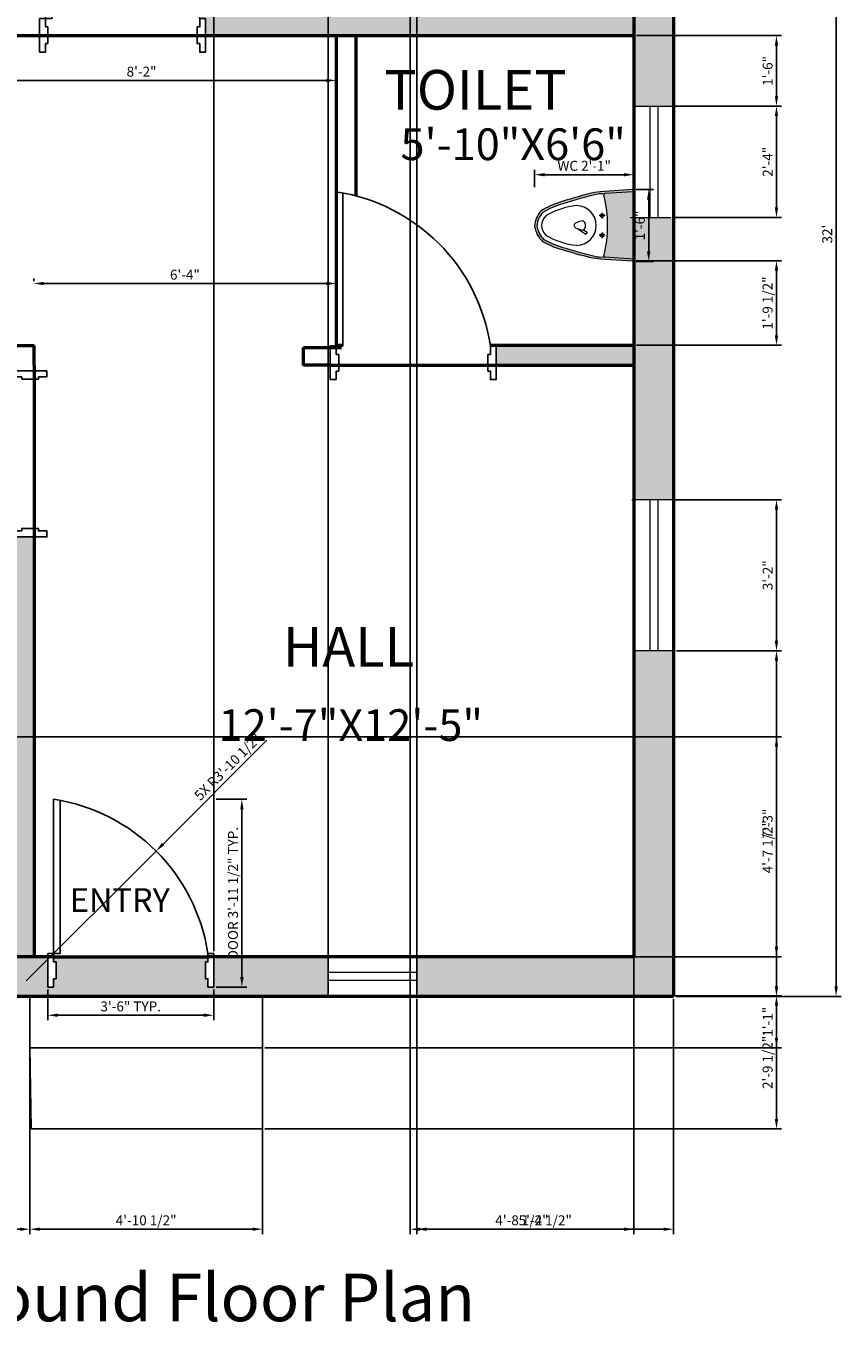
# Model space of a CAD drawing. Units: inches. Extents: x 3578 to 3951, y 1675 to 2189.
# Tile 2 of 4: x 3746 to 3951, y 1675 to 2001. Entities that reach past the tile are written whole.
import ezdxf

# ---------------------------------------------------------------- set-up
doc = ezdxf.new("R2010")
doc.units = ezdxf.units.IN
for name, color, linetype, lineweight in [('A-ANNO-DIMS', 2, 'Continuous', 18), ('A-ANNO-TEXT', 7, 'Continuous', 25), ('A-AREA-IDEN', 7, 'Continuous', 25), ('A-DOOR', 3, 'Continuous', 25), ('A-FLOR-FIXT', 9, 'Continuous', 18), ('A-FLOR-STRS', 7, 'Continuous', 25), ('A-GLAZ', 4, 'Continuous', 18), ('A-WALL', 7, 'Continuous', 50), ('A-WALL-PATT', 8, 'Continuous', 13)]:
    doc.layers.add(name, color=color, linetype=linetype, lineweight=lineweight)
doc.styles.get("Standard").update_dxf_attribs({"font": 'arial.ttf'})
doc.dimstyles.new('ISO-25', dxfattribs={"dimtxt": 2.5, "dimasz": 2.5, "dimexe": 1.25, "dimexo": 0.625, "dimtad": 1, "dimdec": 0, "dimlunit": 4, "dimtxsty": 'Standard', "dimcen": 2.5, "dimadec": 0, "dimazin": 0, "dimtfac": 1, "dimtdec": 0, "dimtmove": 0, "dimatfit": 3, "dimfxl": 1, "dimarcsym": 0})

# ---------------------------------------------------------------- blocks, each defined once
blk = doc.blocks.new('A$C40E8097C')
for p, q in [((33.6, 192), (33.6, 1074.8)), ((72, 192), (72, 1068.3)), ((0, 192), (0, 0)), ((33.6, 192), (0, 192)), ((33.6, 144), (33.6, 192)), ((48, 144), (33.6, 144)), ((48, 48), (48, 144)), ((33.6, 0), (33.6, 48)), ((33.6, 48), (48, 48)), ((0, 0), (33.6, 0))]:
    blk.add_line(p, q)
blk.add_lwpolyline([(33.6, 192), (72, 192)])
blk.add_lwpolyline([(950, 192), (950, 0), (916.4, 0), (916.4, 48), (902, 48), (902, 144), (916.4, 144), (916.4, 192)], close=True)
blk.add_arc((-123.6, 34.8), 1051.8, 8.59637, 81.40363)
blk = doc.blocks.new('A$C43D762ED')
for p, q in [((0, 0.729), (0.0157, 0.4897)), ((0.5246, 0.7397), (0.01, 0.7397)), ((0.0162, 0.7328), (0.0298, 0.5262)), ((0.5184, 0.7328), (0.5048, 0.5262)), ((0.5346, 0.729), (0.5189, 0.4897)), ((0.0157, 0.4897), (0.0223, 0.4455)), ((0.2151, 0.5034), (0.172, 0.5034)), ((0.1938, 0.525), (0.1938, 0.4814)), ((0.3195, 0.5034), (0.3626, 0.5034)), ((0.3408, 0.525), (0.3408, 0.4814)), ((0.5189, 0.4897), (0.5123, 0.4455)), ((0.3001, 0.3651), (0.3169, 0.3911)), ((0.3169, 0.3911), (0.3311, 0.382)), ((0.2923, 0.3214), (0.3311, 0.382)), ((0.0888, 0.2044), (0.0937, 0.19))]:
    blk.add_line(p, q)
for centre in [(0.1938, 0.5034), (0.3408, 0.5034)]:
    blk.add_circle(centre, 0.0137)
for centre, radius, start, end in [((0.01, 0.7297), 0.01, 90, 183.76235), ((0.0257, 0.7297), 0.01, 90, 161.99285), ((0.5089, 0.7297), 0.01, 18.00715, 90), ((0.5246, 0.7297), 0.01, 356.23765, 90), ((0.0398, 0.5269), 0.01, 183.76235, 283.82831), ((0.1268, 0.4939), 0.0953, 165.17281, 194.54705), ((0.2673, -0.3974), 0.9419, 76.14598, 103.82831), ((0.4948, 0.5269), 0.01, 256.17169, 356.23765), ((0.4078, 0.4939), 0.0953, 345.45295, 14.82719), ((2.7485, 1.0673), 2.7962, 192.84784, 197.97333), ((2.7485, 1.0673), 2.7789, 192.41213, 197.97333), ((0.2675, 0.3121), 0.148, 90, 180), ((0.2675, 0.3121), 0.148, 0, 90), ((-2.2139, 1.0673), 2.7789, 342.53599, 347.58787), ((-2.2139, 1.0673), 2.7962, 342.54844, 347.15216), ((0.6936, 0.3754), 0.5775, 186.28683, 210.10499), ((0.2395, 0.3612), 0.006, 139.49966, 184.26121), ((0.3639, 0.3708), 0.1308, 184.40911, 210.02383), ((0.2675, 0.3372), 0.0429, 40.50034, 139.49966), ((0.2721, 0.3185), 0.0252, 211.47881, 259.49934), ((0.2629, 0.3185), 0.0252, 280.50066, 328.52119), ((0.1712, 0.3708), 0.1308, 329.97617, 355.59089), ((0.2956, 0.3612), 0.006, 355.73879, 40.50034), ((-0.1586, 0.3754), 0.5775, 329.89501, 353.71317), ((0.714, 0.3854), 0.6336, 196.09704, 210.8164), ((-0.1586, 0.3754), 0.6121, 329.89501, 346.57808), ((-0.1586, 0.3754), 0.6294, 329.89501, 346.52221), ((0.7246, 0.3908), 0.662, 197.65406, 211.16701), ((0.2834, 0.1859), 0.1862, 227.70774, 266.91661), ((0.2818, 0.1811), 0.1643, 227.04359, 266.25246), ((0.2786, 0.1719), 0.1209, 225.50669, 264.71555), ((0.2564, 0.1719), 0.1209, 275.28445, 314.49331), ((0.2492, 0.183), 0.1673, 277.51863, 316.7275), ((0.2459, 0.188), 0.1899, 278.30562, 317.51449)]:
    blk.add_arc(centre, radius, start, end)
blk = doc.blocks.new('*D11')
at = {"layer": 'A-ANNO-DIMS', "color": 0, "lineweight": -2, "transparency": 16777216}
for p, q in [((3909.8, 2140.77), (3951.35, 2140.77)), ((3950.1, 2138.27), (3950.1, 1759.27)), ((3909.8, 1756.77), (3951.35, 1756.77))]:
    blk.add_line(p, q, dxfattribs=at)
at = {"layer": 'A-ANNO-DIMS', "color": 0, "transparency": 16777216}
for points in [[(3949.68, 2138.27), (3950.51, 2138.27), (3950.1, 2140.77)], [(3949.68, 1759.27), (3950.51, 1759.27), (3950.1, 1756.77)]]:
    blk.add_solid(points, dxfattribs=at)
at = {"layer": 'Defpoints', "color": 0, "transparency": 16777216}
for p in [(3909.18, 2140.77), (3909.18, 1756.77), (3950.1, 1756.77)]:
    blk.add_point(p, dxfattribs=at)
at = {"layer": 'A-ANNO-DIMS', "color": 0, "transparency": 16777216, "insert": (3948.19, 1948.77), "char_height": 2.5, "attachment_point": 5, "rotation": 90}
blk.add_mtext("32'", dxfattribs=at)
blk = doc.blocks.new('*D12')
at = {"layer": 'A-ANNO-DIMS', "color": 0, "lineweight": -2, "transparency": 16777216}
for p, q in [((3726.18, 1987.68), (3726.18, 1986.23)), ((3728.68, 1987.48), (3821.68, 1987.48)), ((3824.18, 1987.68), (3824.18, 1986.23))]:
    blk.add_line(p, q, dxfattribs=at)
at = {"layer": 'A-ANNO-DIMS', "color": 0, "transparency": 16777216}
for points in [[(3728.68, 1987.9), (3728.68, 1987.07), (3726.18, 1987.48)], [(3821.68, 1987.9), (3821.68, 1987.07), (3824.18, 1987.48)]]:
    blk.add_solid(points, dxfattribs=at)
at = {"layer": 'Defpoints', "color": 0, "transparency": 16777216}
for p in [(3726.18, 1988.31), (3824.18, 1988.31), (3824.18, 1987.48)]:
    blk.add_point(p, dxfattribs=at)
at = {"layer": 'A-ANNO-DIMS', "color": 0, "transparency": 16777216, "insert": (3775.18, 1989.38), "char_height": 2.5, "attachment_point": 5}
blk.add_mtext('8\'-2"', dxfattribs=at)
blk = doc.blocks.new('*D13')
at = {"layer": 'A-ANNO-DIMS', "color": 0, "lineweight": -2, "transparency": 16777216}
for p, q in [((3748.01, 1936.96), (3748.01, 1937.58)), ((3821.7, 1936.33), (3750.51, 1936.33)), ((3824.2, 1936.96), (3824.2, 1937.58))]:
    blk.add_line(p, q, dxfattribs=at)
at = {"layer": 'A-ANNO-DIMS', "color": 0, "transparency": 16777216}
for points in [[(3750.51, 1936.75), (3750.51, 1935.92), (3748.01, 1936.33)], [(3821.7, 1936.75), (3821.7, 1935.92), (3824.2, 1936.33)]]:
    blk.add_solid(points, dxfattribs=at)
at = {"layer": 'Defpoints', "color": 0, "transparency": 16777216}
for p in [(3748.01, 1936.33), (3748.01, 1936.33), (3824.2, 1936.33)]:
    blk.add_point(p, dxfattribs=at)
at = {"layer": 'A-ANNO-DIMS', "color": 0, "transparency": 16777216, "insert": (3786.1, 1938.23), "char_height": 2.5, "attachment_point": 5}
blk.add_mtext('6\'-4"', dxfattribs=at)
blk = doc.blocks.new('*D15')
at = {"layer": 'A-ANNO-DIMS', "color": 0, "lineweight": -2, "transparency": 16777216}
for p, q in [((3793.98, 1806.42), (3801.7, 1806.42)), ((3800.45, 1761.62), (3800.45, 1803.92)), ((3793.98, 1759.12), (3801.7, 1759.12))]:
    blk.add_line(p, q, dxfattribs=at)
at = {"layer": 'A-ANNO-DIMS', "color": 0, "transparency": 16777216}
for points in [[(3800.03, 1803.92), (3800.87, 1803.92), (3800.45, 1806.42)], [(3800.03, 1761.62), (3800.87, 1761.62), (3800.45, 1759.12)]]:
    blk.add_solid(points, dxfattribs=at)
at = {"layer": 'Defpoints', "color": 0, "transparency": 16777216}
for p in [(3793.35, 1806.42), (3800.45, 1806.42), (3793.35, 1759.12)]:
    blk.add_point(p, dxfattribs=at)
at = {"layer": 'A-ANNO-DIMS', "color": 0, "transparency": 16777216, "insert": (3798.53, 1782.77), "char_height": 2.5, "attachment_point": 5, "rotation": 90}
blk.add_mtext('DOOR 3\'-11 1/2" TYP.', dxfattribs=at)
blk = doc.blocks.new('*D16')
at = {"layer": 'A-ANNO-DIMS', "color": 0, "lineweight": -2, "transparency": 16777216}
for p, q in [((3751.55, 1758.49), (3751.55, 1750.77)), ((3793.35, 1758.49), (3793.35, 1750.77)), ((3754.05, 1752.02), (3790.85, 1752.02))]:
    blk.add_line(p, q, dxfattribs=at)
at = {"layer": 'A-ANNO-DIMS', "color": 0, "transparency": 16777216}
for points in [[(3754.05, 1752.44), (3754.05, 1751.61), (3751.55, 1752.02)], [(3790.85, 1752.44), (3790.85, 1751.61), (3793.35, 1752.02)]]:
    blk.add_solid(points, dxfattribs=at)
at = {"layer": 'Defpoints', "color": 0, "transparency": 16777216}
for p in [(3751.55, 1759.12), (3793.35, 1759.12), (3793.35, 1752.02)]:
    blk.add_point(p, dxfattribs=at)
at = {"layer": 'A-ANNO-DIMS', "color": 0, "transparency": 16777216, "insert": (3772.45, 1753.92), "char_height": 2.5, "attachment_point": 5}
blk.add_mtext('3\'-6" TYP.', dxfattribs=at)
blk = doc.blocks.new('*D21')
at = {"layer": 'A-ANNO-DIMS', "color": 0, "lineweight": -2, "transparency": 16777216}
for p, q in [((3874.16, 1960.61), (3874.16, 1964.98)), ((3876.66, 1963.73), (3896.65, 1963.73)), ((3899.15, 1960.61), (3899.15, 1964.98))]:
    blk.add_line(p, q, dxfattribs=at)
at = {"layer": 'A-ANNO-DIMS', "color": 0, "transparency": 16777216}
for points in [[(3876.66, 1964.15), (3876.66, 1963.32), (3874.16, 1963.73)], [(3896.65, 1964.15), (3896.65, 1963.32), (3899.15, 1963.73)]]:
    blk.add_solid(points, dxfattribs=at)
at = {"layer": 'Defpoints', "color": 0, "transparency": 16777216}
for p in [(3899.15, 1963.73), (3874.16, 1959.99), (3899.15, 1959.99)]:
    blk.add_point(p, dxfattribs=at)
at = {"layer": 'A-ANNO-DIMS', "color": 0, "transparency": 16777216, "insert": (3886.66, 1965.65), "char_height": 2.5, "attachment_point": 5}
blk.add_mtext('WC 2\'-1"', dxfattribs=at)
blk = doc.blocks.new('*D22')
at = {"layer": 'A-ANNO-DIMS', "color": 0, "lineweight": -2, "transparency": 16777216}
for p, q in [((3899.77, 1959.99), (3904.15, 1959.99)), ((3902.9, 1957.49), (3902.9, 1944.41)), ((3899.77, 1941.91), (3904.15, 1941.91))]:
    blk.add_line(p, q, dxfattribs=at)
at = {"layer": 'A-ANNO-DIMS', "color": 0, "transparency": 16777216}
for points in [[(3902.48, 1957.49), (3903.31, 1957.49), (3902.9, 1959.99)], [(3902.48, 1944.41), (3903.31, 1944.41), (3902.9, 1941.91)]]:
    blk.add_solid(points, dxfattribs=at)
at = {"layer": 'Defpoints', "color": 0, "transparency": 16777216}
for p in [(3899.15, 1959.99), (3899.15, 1941.91), (3902.9, 1941.91)]:
    blk.add_point(p, dxfattribs=at)
at = {"layer": 'A-ANNO-DIMS', "color": 0, "transparency": 16777216, "insert": (3901, 1950.95), "char_height": 2.5, "attachment_point": 5, "rotation": 90}
blk.add_mtext('1\'-6"', dxfattribs=at)
blk = doc.blocks.new('*D33')
at = {"layer": 'A-ANNO-DIMS', "color": 0, "lineweight": -2, "transparency": 16777216}
for p, q in [((3899.8, 1998.77), (3936.33, 1998.77)), ((3935.08, 1996.27), (3935.08, 1983.49)), ((3909.48, 1980.99), (3936.33, 1980.99))]:
    blk.add_line(p, q, dxfattribs=at)
at = {"layer": 'A-ANNO-DIMS', "color": 0, "transparency": 16777216}
for points in [[(3934.66, 1996.27), (3935.5, 1996.27), (3935.08, 1998.77)], [(3934.66, 1983.49), (3935.5, 1983.49), (3935.08, 1980.99)]]:
    blk.add_solid(points, dxfattribs=at)
at = {"layer": 'Defpoints', "color": 0, "transparency": 16777216}
for p in [(3899.18, 1998.77), (3908.86, 1980.99), (3935.08, 1980.99)]:
    blk.add_point(p, dxfattribs=at)
at = {"layer": 'A-ANNO-DIMS', "color": 0, "transparency": 16777216, "insert": (3933.18, 1989.88), "char_height": 2.5, "attachment_point": 5, "rotation": 90}
blk.add_mtext('1\'-6"', dxfattribs=at)
blk = doc.blocks.new('*D34')
at = {"layer": 'A-ANNO-DIMS', "color": 0, "lineweight": -2, "transparency": 16777216}
for p, q in [((3909.48, 1980.99), (3936.33, 1980.99)), ((3935.08, 1978.49), (3935.08, 1955.48)), ((3909.11, 1952.98), (3936.33, 1952.98))]:
    blk.add_line(p, q, dxfattribs=at)
at = {"layer": 'A-ANNO-DIMS', "color": 0, "transparency": 16777216}
for points in [[(3934.66, 1978.49), (3935.5, 1978.49), (3935.08, 1980.99)], [(3934.66, 1955.48), (3935.5, 1955.48), (3935.08, 1952.98)]]:
    blk.add_solid(points, dxfattribs=at)
at = {"layer": 'Defpoints', "color": 0, "transparency": 16777216}
for p in [(3908.86, 1980.99), (3908.48, 1952.98), (3935.08, 1952.98)]:
    blk.add_point(p, dxfattribs=at)
at = {"layer": 'A-ANNO-DIMS', "color": 0, "transparency": 16777216, "insert": (3933.2, 1966.99), "char_height": 2.5, "attachment_point": 5, "rotation": 90}
blk.add_mtext('2\'-4"', dxfattribs=at)
blk = doc.blocks.new('*D35')
at = {"layer": 'A-ANNO-DIMS', "color": 0, "lineweight": -2, "transparency": 16777216}
for p, q in [((3909.92, 1843.84), (3936.33, 1843.84)), ((3935.08, 1759.27), (3935.08, 1841.34)), ((3909.8, 1756.77), (3936.33, 1756.77))]:
    blk.add_line(p, q, dxfattribs=at)
at = {"layer": 'A-ANNO-DIMS', "color": 0, "transparency": 16777216}
for points in [[(3934.66, 1841.34), (3935.5, 1841.34), (3935.08, 1843.84)], [(3934.66, 1759.27), (3935.5, 1759.27), (3935.08, 1756.77)]]:
    blk.add_solid(points, dxfattribs=at)
at = {"layer": 'Defpoints', "color": 0, "transparency": 16777216}
for p in [(3909.3, 1843.84), (3935.08, 1843.84), (3909.18, 1756.77)]:
    blk.add_point(p, dxfattribs=at)
at = {"layer": 'A-ANNO-DIMS', "color": 0, "transparency": 16777216, "insert": (3933.18, 1800.3), "char_height": 2.5, "attachment_point": 5, "rotation": 90}
blk.add_mtext('7\'-3"', dxfattribs=at)
blk = doc.blocks.new('*D36')
at = {"layer": 'A-ANNO-DIMS', "color": 0, "lineweight": -2, "transparency": 16777216}
for p, q in [((3909.61, 1881.86), (3936.33, 1881.86)), ((3935.08, 1879.36), (3935.08, 1846.34)), ((3909.92, 1843.84), (3936.33, 1843.84))]:
    blk.add_line(p, q, dxfattribs=at)
at = {"layer": 'A-ANNO-DIMS', "color": 0, "transparency": 16777216}
for points in [[(3934.66, 1879.36), (3935.5, 1879.36), (3935.08, 1881.86)], [(3934.66, 1846.34), (3935.5, 1846.34), (3935.08, 1843.84)]]:
    blk.add_solid(points, dxfattribs=at)
at = {"layer": 'Defpoints', "color": 0, "transparency": 16777216}
for p in [(3908.98, 1881.86), (3909.3, 1843.84), (3935.08, 1843.84)]:
    blk.add_point(p, dxfattribs=at)
at = {"layer": 'A-ANNO-DIMS', "color": 0, "transparency": 16777216, "insert": (3933.18, 1862.85), "char_height": 2.5, "attachment_point": 5, "rotation": 90}
blk.add_mtext('3\'-2"', dxfattribs=at)
blk = doc.blocks.new('*D39')
at = {"layer": 'A-ANNO-DIMS', "color": 0, "lineweight": -2, "transparency": 16777216}
for p, q in [((3685.29, 1756.14), (3685.29, 1696.88)), ((3747.04, 1756.14), (3747.04, 1696.88)), ((3687.79, 1698.13), (3744.54, 1698.13))]:
    blk.add_line(p, q, dxfattribs=at)
at = {"layer": 'A-ANNO-DIMS', "color": 0, "transparency": 16777216}
for points in [[(3687.79, 1698.55), (3687.79, 1697.71), (3685.29, 1698.13)], [(3744.54, 1698.55), (3744.54, 1697.71), (3747.04, 1698.13)]]:
    blk.add_solid(points, dxfattribs=at)
at = {"layer": 'Defpoints', "color": 0, "transparency": 16777216}
for p in [(3685.29, 1756.77), (3747.04, 1756.77), (3747.04, 1698.13)]:
    blk.add_point(p, dxfattribs=at)
at = {"layer": 'A-ANNO-DIMS', "color": 0, "transparency": 16777216, "insert": (3716.16, 1700.05), "char_height": 2.5, "attachment_point": 5}
blk.add_mtext('5\'-1 1/2"', dxfattribs=at)
blk = doc.blocks.new('*D40')
at = {"layer": 'A-ANNO-DIMS', "color": 0, "lineweight": -2, "transparency": 16777216}
for p, q in [((3747.04, 1756.14), (3747.04, 1696.88)), ((3805.63, 1756.3), (3805.63, 1696.88)), ((3749.54, 1698.13), (3803.13, 1698.13))]:
    blk.add_line(p, q, dxfattribs=at)
at = {"layer": 'A-ANNO-DIMS', "color": 0, "transparency": 16777216}
for points in [[(3749.54, 1698.55), (3749.54, 1697.71), (3747.04, 1698.13)], [(3803.13, 1698.55), (3803.13, 1697.71), (3805.63, 1698.13)]]:
    blk.add_solid(points, dxfattribs=at)
at = {"layer": 'Defpoints', "color": 0, "transparency": 16777216}
for p in [(3747.04, 1756.77), (3805.63, 1756.92), (3805.63, 1698.13)]:
    blk.add_point(p, dxfattribs=at)
at = {"layer": 'A-ANNO-DIMS', "color": 0, "transparency": 16777216, "insert": (3776.33, 1700.05), "char_height": 2.5, "attachment_point": 5}
blk.add_mtext('4\'-10 1/2"', dxfattribs=at)
blk = doc.blocks.new('*D41')
at = {"layer": 'A-ANNO-DIMS', "color": 0, "lineweight": -2, "transparency": 16777216}
for p, q in [((3806.26, 1756.92), (3936.33, 1756.92)), ((3935.08, 1725.88), (3935.08, 1754.42)), ((3806.26, 1723.38), (3936.33, 1723.38))]:
    blk.add_line(p, q, dxfattribs=at)
at = {"layer": 'A-ANNO-DIMS', "color": 0, "transparency": 16777216}
for points in [[(3934.66, 1754.42), (3935.5, 1754.42), (3935.08, 1756.92)], [(3934.66, 1725.88), (3935.5, 1725.88), (3935.08, 1723.38)]]:
    blk.add_solid(points, dxfattribs=at)
at = {"layer": 'Defpoints', "color": 0, "transparency": 16777216}
for p in [(3805.63, 1756.92), (3935.08, 1756.92), (3805.63, 1723.38)]:
    blk.add_point(p, dxfattribs=at)
at = {"layer": 'A-ANNO-DIMS', "color": 0, "transparency": 16777216, "insert": (3933.16, 1740.15), "char_height": 2.5, "attachment_point": 5, "rotation": 90}
blk.add_mtext('2\'-9 1/2"', dxfattribs=at)
blk = doc.blocks.new('*D42')
at = {"layer": 'A-ANNO-DIMS', "color": 0, "lineweight": -2, "transparency": 16777216}
for p, q in [((3806.26, 1756.92), (3936.33, 1756.92)), ((3935.08, 1746.31), (3935.08, 1754.42)), ((3806.26, 1743.81), (3936.33, 1743.81))]:
    blk.add_line(p, q, dxfattribs=at)
at = {"layer": 'A-ANNO-DIMS', "color": 0, "transparency": 16777216}
for points in [[(3934.66, 1754.42), (3935.5, 1754.42), (3935.08, 1756.92)], [(3934.66, 1746.31), (3935.5, 1746.31), (3935.08, 1743.81)]]:
    blk.add_solid(points, dxfattribs=at)
at = {"layer": 'Defpoints', "color": 0, "transparency": 16777216}
for p in [(3805.63, 1756.92), (3935.08, 1756.92), (3805.63, 1743.81)]:
    blk.add_point(p, dxfattribs=at)
at = {"layer": 'A-ANNO-DIMS', "color": 0, "transparency": 16777216, "insert": (3933.2, 1750.37), "char_height": 2.5, "attachment_point": 5, "rotation": 90}
blk.add_mtext('1\'-1"', dxfattribs=at)
blk = doc.blocks.new('*D43')
at = {"layer": 'A-ANNO-DIMS', "color": 0, "lineweight": -2, "transparency": 16777216}
for p, q in [((3822.14, 1757.39), (3822.14, 2167.33)), ((3824.64, 2166.08), (3841.99, 2166.08)), ((3844.49, 1757.39), (3844.49, 2167.33))]:
    blk.add_line(p, q, dxfattribs=at)
at = {"layer": 'A-ANNO-DIMS', "color": 0, "transparency": 16777216}
for points in [[(3824.64, 2166.49), (3824.64, 2165.66), (3822.14, 2166.08)], [(3841.99, 2166.49), (3841.99, 2165.66), (3844.49, 2166.08)]]:
    blk.add_solid(points, dxfattribs=at)
at = {"layer": 'Defpoints', "color": 0, "transparency": 16777216}
for p in [(3844.49, 2166.08), (3822.14, 1756.77), (3844.49, 1756.77)]:
    blk.add_point(p, dxfattribs=at)
at = {"layer": 'A-ANNO-DIMS', "color": 0, "transparency": 16777216, "insert": (3833.31, 2167.99), "char_height": 2.5, "attachment_point": 5}
blk.add_mtext('1\'-10 1/2"', dxfattribs=at)
blk = doc.blocks.new('*D44')
at = {"layer": 'A-ANNO-DIMS', "color": 0, "lineweight": -2, "transparency": 16777216}
for p, q in [((3844.49, 1756.14), (3844.49, 1696.88)), ((3909.18, 1756.14), (3909.18, 1696.88)), ((3846.99, 1698.13), (3906.68, 1698.13))]:
    blk.add_line(p, q, dxfattribs=at)
at = {"layer": 'A-ANNO-DIMS', "color": 0, "transparency": 16777216}
for points in [[(3846.99, 1698.55), (3846.99, 1697.71), (3844.49, 1698.13)], [(3906.68, 1698.55), (3906.68, 1697.71), (3909.18, 1698.13)]]:
    blk.add_solid(points, dxfattribs=at)
at = {"layer": 'Defpoints', "color": 0, "transparency": 16777216}
for p in [(3844.49, 1756.77), (3909.18, 1756.77), (3909.18, 1698.13)]:
    blk.add_point(p, dxfattribs=at)
at = {"layer": 'A-ANNO-DIMS', "color": 0, "transparency": 16777216, "insert": (3876.84, 1700.05), "char_height": 2.5, "attachment_point": 5}
blk.add_mtext('5\'-4 1/2"', dxfattribs=at)
blk = doc.blocks.new('*D51')
at = {"layer": 'A-ANNO-DIMS', "color": 0, "lineweight": -2, "transparency": 16777216}
for p, q in [((3899.71, 1942.06), (3936.33, 1942.06)), ((3935.08, 1923.27), (3935.08, 1939.56)), ((3899.8, 1920.77), (3936.33, 1920.77))]:
    blk.add_line(p, q, dxfattribs=at)
at = {"layer": 'A-ANNO-DIMS', "color": 0, "transparency": 16777216}
for points in [[(3934.66, 1939.56), (3935.5, 1939.56), (3935.08, 1942.06)], [(3934.66, 1923.27), (3935.5, 1923.27), (3935.08, 1920.77)]]:
    blk.add_solid(points, dxfattribs=at)
at = {"layer": 'Defpoints', "color": 0, "transparency": 16777216}
for p in [(3899.09, 1942.06), (3935.08, 1942.06), (3899.18, 1920.77)]:
    blk.add_point(p, dxfattribs=at)
at = {"layer": 'A-ANNO-DIMS', "color": 0, "transparency": 16777216, "insert": (3933.16, 1931.41), "char_height": 2.5, "attachment_point": 5, "rotation": 90}
blk.add_mtext('1\'-9 1/2"', dxfattribs=at)
blk = doc.blocks.new('*D56')
at = {"layer": 'A-ANNO-DIMS', "color": 0, "lineweight": -2, "transparency": 16777216}
for p, q in [((3842.79, 2129.55), (3842.79, 1696.88)), ((3899.18, 2130.14), (3899.18, 1696.88)), ((3896.68, 1698.13), (3845.29, 1698.13))]:
    blk.add_line(p, q, dxfattribs=at)
at = {"layer": 'A-ANNO-DIMS', "color": 0, "transparency": 16777216}
for points in [[(3845.29, 1698.55), (3845.29, 1697.71), (3842.79, 1698.13)], [(3896.68, 1698.55), (3896.68, 1697.71), (3899.18, 1698.13)]]:
    blk.add_solid(points, dxfattribs=at)
at = {"layer": 'Defpoints', "color": 0, "transparency": 16777216}
for p in [(3842.79, 2130.17), (3899.18, 2130.77), (3842.79, 1698.13)]:
    blk.add_point(p, dxfattribs=at)
at = {"layer": 'A-ANNO-DIMS', "color": 0, "transparency": 16777216, "insert": (3870.98, 1700.05), "char_height": 2.5, "attachment_point": 5}
blk.add_mtext('4\'-8 1/2"', dxfattribs=at)
blk = doc.blocks.new('*D57')
at = {"layer": 'A-ANNO-DIMS', "color": 0, "lineweight": -2, "transparency": 16777216}
for p, q in [((3620.74, 1822.18), (3936.33, 1822.18)), ((3935.08, 1769.27), (3935.08, 1819.68)), ((3619.8, 1766.77), (3936.33, 1766.77))]:
    blk.add_line(p, q, dxfattribs=at)
at = {"layer": 'A-ANNO-DIMS', "color": 0, "transparency": 16777216}
for points in [[(3934.66, 1819.68), (3935.5, 1819.68), (3935.08, 1822.18)], [(3934.66, 1769.27), (3935.5, 1769.27), (3935.08, 1766.77)]]:
    blk.add_solid(points, dxfattribs=at)
at = {"layer": 'Defpoints', "color": 0, "transparency": 16777216}
for p in [(3620.11, 1822.18), (3935.08, 1822.18), (3619.18, 1766.77)]:
    blk.add_point(p, dxfattribs=at)
at = {"layer": 'A-ANNO-DIMS', "color": 0, "transparency": 16777216, "insert": (3933.16, 1794.47), "char_height": 2.5, "attachment_point": 5, "rotation": 90}
blk.add_mtext('4\'-7 1/2"', dxfattribs=at)
blk = doc.blocks.new('*D59')
at = {"layer": 'A-ANNO-DIMS', "color": 0, "lineweight": -2, "transparency": 16777216}
for p, q in [((3793.35, 1768.19), (3793.35, 2167.33)), ((3795.85, 2166.08), (3819.64, 2166.08)), ((3822.14, 1767.4), (3822.14, 2167.33))]:
    blk.add_line(p, q, dxfattribs=at)
at = {"layer": 'A-ANNO-DIMS', "color": 0, "transparency": 16777216}
for points in [[(3795.85, 2166.49), (3795.85, 2165.66), (3793.35, 2166.08)], [(3819.64, 2166.49), (3819.64, 2165.66), (3822.14, 2166.08)]]:
    blk.add_solid(points, dxfattribs=at)
at = {"layer": 'Defpoints', "color": 0, "transparency": 16777216}
for p in [(3822.14, 2166.08), (3793.35, 1767.57), (3822.14, 1766.77)]:
    blk.add_point(p, dxfattribs=at)
at = {"layer": 'A-ANNO-DIMS', "color": 0, "transparency": 16777216, "insert": (3807.75, 2167.98), "char_height": 2.5, "attachment_point": 5}
blk.add_mtext('2\'-5"', dxfattribs=at)
blk = doc.blocks.new('*D60')
at = {"layer": 'A-ANNO-DIMS', "color": 0, "lineweight": -2, "transparency": 16777216}
for p, q in [((3806.76, 1821.3), (3780.61, 1795.15)), ((3746.11, 1760.65), (3778.84, 1793.38))]:
    blk.add_line(p, q, dxfattribs=at)
at = {"layer": 'A-ANNO-DIMS', "color": 0, "transparency": 16777216}
blk.add_solid([(3780.31, 1795.44), (3780.9, 1794.85), (3778.84, 1793.38)], dxfattribs=at)
at = {"layer": 'Defpoints', "color": 0, "transparency": 16777216}
for p in [(3778.84, 1793.38), (3746.11, 1760.65)]:
    blk.add_point(p, dxfattribs=at)
at = {"layer": 'A-ANNO-DIMS', "color": 0, "transparency": 16777216, "insert": (3797.12, 1814.37), "char_height": 2.5, "attachment_point": 5, "rotation": 44.9999}
blk.add_mtext('5X R3\'-10 1/2"', dxfattribs=at)

msp = doc.modelspace()

# ---------------------------------------------------------------- hatches: boundary and pattern name
at = {"layer": 'A-WALL-PATT'}
h = msp.add_hatch(color=256, dxfattribs=at)
h.dxf.hatch_style = 1
h.paths.add_polyline_path([(3619.18, 1950.71), (3609.18, 1950.71), (3609.18, 1756.77), (3648.78, 1756.77), (3648.78, 1766.77), (3619.18, 1766.77)])
h.paths.add_polyline_path([(3619.18, 2068.71), (3609.18, 2068.71), (3609.18, 1975.57), (3619.18, 1975.57), (3619.18, 1998.77)])
h.paths.add_polyline_path([(3619.18, 2130.77), (3647.07, 2130.77), (3647.07, 2140.77), (3609.18, 2140.77), (3609.18, 2104.48), (3619.18, 2104.48)])
h.paths.add_polyline_path([(3909.18, 2140.77), (3713.13, 2140.77), (3713.13, 2130.77), (3899.18, 2130.77), (3899.18, 2110.42), (3909.18, 2110.42)])
h.paths.add_polyline_path([(3909.18, 2050.5), (3899.18, 2050.5), (3899.18, 1980.99), (3909.18, 1980.99)])
h.paths.add_polyline_path([(3909.18, 1881.86), (3899.18, 1881.86), (3899.18, 1941.89), (3890.7, 1942.45), (3889.21, 1942.68, -0.02009), (3881.89, 1944.66, -0.072677), (3876.18, 1946.94, -0.17277), (3874.16, 1950.75, -0.17277), (3875.79, 1954.64, -0.055418), (3880.27, 1956.72, -0.024581), (3889.21, 1959.22), (3890.7, 1959.45), (3899.18, 1960.01), (3899.18, 1952.98), (3909.18, 1952.98)])
h.paths.add_polyline_path([(3891.56, 1958.83, 0.100666), (3890.28, 1958.86, 0.024932), (3881.25, 1956.42, 0.064314), (3876.22, 1954.24, 0.17277), (3874.74, 1950.82, 0.17277), (3876.47, 1947.45, 0.072922), (3882.04, 1945.22, 0.022708), (3890.28, 1943.04, 0.100666), (3891.56, 1943.07, 0.125847)], flags=16)
h.paths.add_polyline_path([(3898.92, 1942.47, 0.324885), (3899.15, 1942.79), (3899.15, 1959.11, 0.551642), (3898.67, 1959.41), (3899.15, 1959.45), (3899.15, 1942.45)], flags=16)
h.paths.add_polyline_path([(3890.7, 1948.47, -1), (3891.63, 1948.47, -1)], flags=0)
h.paths.add_polyline_path([(3884.71, 1945.94, -0.104302), (3877.06, 1948.46, -0.17277), (3875.9, 1950.94, -0.17277), (3877.06, 1953.43, -0.104302), (3884.71, 1955.94, -0.414214), (3889.71, 1950.94, -0.414214)], flags=0)
h.paths.add_polyline_path([(3887.07, 1948.79), (3885.02, 1950.11, -0.031181), (3884.52, 1950.35, -0.229141), (3884.09, 1950.94, -0.229141), (3884.52, 1951.54, -0.109107), (3886.35, 1952.09, -0.199237), (3886.5, 1952.04, -0.461153), (3886.5, 1949.84), (3887.38, 1949.28)], flags=0)
h.paths.add_polyline_path([(3890.7, 1953.43, -1), (3891.63, 1953.43, -1)], flags=0)
h.paths.add_polyline_path([(3909.18, 1843.84), (3899.18, 1843.84), (3899.18, 1766.77), (3844.49, 1766.77), (3844.49, 1756.77), (3909.18, 1756.77)])
h = msp.add_hatch(color=256, dxfattribs=at)
h.dxf.hatch_style = 1
h.paths.add_polyline_path([(3899.18, 2003.77), (3789.71, 2003.77, -0.003692), (3789.81, 2003.09), (3791.29, 2003.09), (3791.29, 1998.77), (3899.18, 1998.77)])
h.paths.add_polyline_path([(3748.18, 2130.77), (3743.18, 2130.77), (3743.18, 2003.77), (3748.18, 2003.77)])
h.paths.add_polyline_path([(3899.18, 1920.77), (3864.53, 1920.77), (3864.53, 1915.77), (3899.18, 1915.77)], flags=0)
h.paths.add_polyline_path([(3748.18, 1872.53), (3743.18, 1872.53), (3743.18, 1766.77), (3748.18, 1766.77)], flags=0)
h.paths.add_polyline_path([(3807.15, 1834.35), (3847.1, 1834.35), (3847.1, 1854.95), (3807.15, 1854.95)], flags=8)
h.paths.add_polyline_path([(3791.36, 1816.7), (3859.75, 1816.7), (3859.75, 1833.18), (3791.36, 1833.18)], flags=8)
h.paths.add_polyline_path([(3771.09, 1986.79), (3779.29, 1986.79), (3779.29, 1991.94), (3771.09, 1991.94)], flags=8)
h.paths.add_polyline_path([(3782.02, 1935.64), (3790.22, 1935.64), (3790.22, 1940.79), (3782.02, 1940.79)], flags=8)
h = msp.add_hatch(color=256, dxfattribs=at)
h.dxf.hatch_style = 1
h.paths.add_polyline_path([(3748.18, 1872.53), (3743.18, 1872.53), (3743.18, 1766.77), (3748.18, 1766.77)], flags=0)
h.paths.add_polyline_path([(3815.97, 1920.2), (3822.72, 1920.2), (3822.72, 1920.6), (3824.18, 1920.6), (3824.18, 1998.77), (3791.29, 1998.77), (3791.29, 1994.64), (3789.81, 1994.64), (3789.81, 1996.75), (3789.18, 1996.75), (3789.18, 1998.77), (3751.6, 1998.77), (3751.6, 1996.75), (3750.96, 1996.75), (3750.96, 1994.64), (3749.49, 1994.64), (3749.49, 1998.77), (3741.62, 1998.77), (3741.62, 1995.21), (3740.14, 1995.21), (3740.14, 1997.32), (3739.51, 1997.32), (3739.51, 1998.77), (3726.18, 1998.77), (3726.18, 1920.73), (3726.07, 1920.73), (3619.18, 1920.77), (3619.18, 1915.77), (3743.18, 1915.77), (3743.18, 1914.33), (3751.33, 1914.33), (3751.33, 1912.86), (3749.22, 1912.86), (3749.22, 1912.22), (3745, 1912.22), (3745, 1912.86), (3742.88, 1912.86), (3742.88, 1911.17), (3704.32, 1911.17, 0.31859), (3742.88, 1874.01), (3745, 1874.01), (3745, 1874.64), (3749.22, 1874.64), (3749.22, 1874.01), (3751.33, 1874.01), (3751.33, 1872.53), (3748.18, 1872.53), (3748.18, 1766.77), (3751.55, 1766.77), (3751.55, 1767.57), (3753.03, 1767.57), (3753.03, 1806.42, -0.328818), (3791.88, 1767.57), (3793.35, 1767.57), (3793.35, 1766.77), (3899.18, 1766.77), (3899.18, 1915.77), (3864.53, 1915.77), (3864.53, 1912.15), (3863.05, 1912.15), (3863.05, 1914.26), (3862.42, 1914.26), (3862.42, 1915.77), (3824.84, 1915.77), (3824.84, 1914.26), (3824.2, 1914.26), (3824.2, 1912.15), (3822.72, 1912.15), (3822.72, 1915.77), (3815.97, 1915.77)], flags=17)
h.paths.add_polyline_path([(3815.97, 1920.2), (3822.72, 1920.2), (3822.72, 1920.6), (3824.18, 1920.6), (3824.18, 1998.77), (3791.29, 1998.77), (3791.29, 1994.64), (3789.81, 1994.64), (3789.81, 1996.75), (3789.18, 1996.75), (3789.18, 1998.77), (3751.6, 1998.77), (3751.6, 1996.75), (3750.96, 1996.75), (3750.96, 1994.64), (3749.49, 1994.64), (3749.49, 1998.77), (3741.62, 1998.77), (3741.62, 1995.21), (3740.14, 1995.21), (3740.14, 1997.32), (3739.51, 1997.32), (3739.51, 1998.77), (3726.18, 1998.77), (3726.18, 1920.73), (3619.18, 1920.77), (3619.18, 1915.77), (3743.18, 1915.77), (3743.18, 1914.33), (3751.33, 1914.33), (3751.33, 1912.86), (3749.22, 1912.86), (3749.22, 1912.22), (3745, 1912.22), (3745, 1912.86), (3742.88, 1912.86), (3742.88, 1911.17), (3704.32, 1911.17, 0.31859), (3742.88, 1874.01), (3745, 1874.01), (3745, 1874.64), (3749.22, 1874.64), (3749.22, 1874.01), (3751.33, 1874.01), (3751.33, 1872.53), (3748.18, 1872.53), (3748.18, 1766.77), (3751.55, 1766.77), (3751.55, 1767.57), (3753.03, 1767.57), (3753.03, 1806.42, -0.328818), (3791.88, 1767.57), (3793.35, 1767.57), (3793.35, 1766.77), (3899.18, 1766.77), (3899.18, 1915.77), (3864.53, 1915.77), (3864.53, 1912.15), (3863.05, 1912.15), (3863.05, 1914.26), (3862.42, 1914.26), (3862.42, 1915.77), (3824.84, 1915.77), (3824.84, 1914.26), (3824.2, 1914.26), (3824.2, 1912.15), (3822.72, 1912.15), (3822.72, 1915.77), (3815.97, 1915.77)], flags=17)
h.paths.add_polyline_path([(3699.81, 2003.77), (3619.18, 2003.77), (3619.18, 1998.77), (3699.81, 1998.77)])
h.paths.add_polyline_path([(3807.15, 1834.35), (3847.1, 1834.35), (3847.1, 1854.95), (3807.15, 1854.95)], flags=8)
h.paths.add_polyline_path([(3791.36, 1816.7), (3859.75, 1816.7), (3859.75, 1833.18), (3791.36, 1833.18)], flags=8)
h = msp.add_hatch(color=256, dxfattribs=at)
h.dxf.hatch_style = 1
h.paths.add_polyline_path([(3899.18, 1920.77), (3864.53, 1920.77), (3864.53, 1915.77), (3899.18, 1915.77)])
h = msp.add_hatch(color=256, dxfattribs=at)
h.dxf.hatch_style = 1
h.paths.add_polyline_path([(3748.18, 1872.53), (3743.18, 1872.53), (3743.18, 1766.77), (3748.18, 1766.77)])
h = msp.add_hatch(color=256, dxfattribs=at)
h.dxf.hatch_style = 1
h.paths.add_polyline_path([(3791.24, 1765.45), (3791.88, 1765.45), (3791.88, 1766.77), (3753.03, 1766.77), (3753.03, 1765.45), (3753.66, 1765.45), (3753.66, 1761.23), (3753.03, 1761.23), (3753.03, 1759.12), (3751.55, 1759.12), (3751.55, 1766.77), (3685.29, 1766.77), (3685.29, 1756.77), (3822.14, 1756.77), (3822.14, 1766.77), (3793.35, 1766.77), (3793.35, 1759.12), (3791.88, 1759.12), (3791.88, 1761.23), (3791.24, 1761.23)])

# ---------------------------------------------------------------- linework, layer by layer
at = {"layer": 'A-FLOR-STRS'}
for p, q in [((3747.04, 1756.77), (3747.04, 1743.81)), ((3805.63, 1743.81), (3805.63, 1756.92)), ((3805.63, 1756.92), (3805.63, 1723.38)), ((3747.04, 1743.81), (3805.63, 1743.81)), ((3747.04, 1743.81), (3747.34, 1723.38)), ((3805.63, 1723.38), (3747.34, 1723.38))]:
    msp.add_line(p, q, dxfattribs=at)
at = {"layer": 'A-GLAZ'}
for p, q in [((3899.23, 1980.99), (3908.86, 1980.99)), ((3903.18, 1980.99), (3903.18, 1952.98)), ((3905.18, 1980.99), (3905.18, 1952.98)), ((3898.3, 1952.98), (3908.48, 1952.98)), ((3908.98, 1881.86), (3898.61, 1881.86)), ((3903.18, 1881.86), (3903.18, 1843.84)), ((3905.18, 1881.86), (3905.18, 1843.84)), ((3909.3, 1843.84), (3899.18, 1843.84)), ((3822.14, 1756.77), (3822.14, 1766.77)), ((3844.49, 1756.77), (3844.49, 1766.84)), ((3844.49, 1762.77), (3822.14, 1762.77)), ((3844.49, 1760.77), (3822.14, 1760.77)), ((3844.58, 1760.77), (3822.19, 1760.77))]:
    msp.add_line(p, q, dxfattribs=at)
at = {"layer": 'A-WALL'}
for p, q in [((3909.18, 2140.77), (3909.18, 1756.77)), ((3899.18, 2130.77), (3899.18, 1766.77)), ((3619.18, 1998.77), (3899.18, 1998.77)), ((3824.18, 1998.77), (3824.18, 1920.77)), ((3829.18, 1998.77), (3829.18, 1958.41)), ((3726.07, 1920.73), (3748.16, 1920.73)), ((3748.16, 1915.74), (3748.16, 1920.73)), ((3815.97, 1915.71), (3815.97, 1920.2)), ((3815.97, 1920.2), (3825.5, 1920.2)), ((3824.18, 1920.77), (3825.89, 1920.77)), ((3824.18, 1920.77), (3825.89, 1920.77)), ((3824.18, 1920.77), (3825.89, 1920.77)), ((3863.03, 1920.77), (3899.18, 1920.77)), ((3748.18, 1766.77), (3748.18, 1915.77)), ((3822.72, 1915.77), (3815.97, 1915.77)), ((3822.72, 1915.77), (3899.18, 1915.77)), ((3753.03, 1766.77), (3619.18, 1766.77)), ((3753.03, 1766.77), (3791.88, 1766.77)), ((3899.18, 1766.77), (3791.88, 1766.77)), ((3909.18, 1756.77), (3609.18, 1756.77))]:
    msp.add_line(p, q, dxfattribs=at)

# ---------------------------------------------------------------- block references
at = {"layer": 'A-DOOR', "xscale": 0.044006868052547, "yscale": 0.044006868052547, "zscale": 0.044006868052547}
for p in [(3749.49, 1994.64), (3822.72, 1912.15), (3751.55, 1759.12)]:
    msp.add_blockref('A$C40E8097C', p, dxfattribs=at)
at = {"layer": 'A-DOOR', "xscale": -0.044006868052547, "yscale": 0.044006868052547, "zscale": 0.044006868052547, "rotation": 90}
msp.add_blockref('A$C40E8097C', (3751.33, 1914.33), dxfattribs=at)
at = {"layer": 'A-FLOR-FIXT', "xscale": 33.78088138767845, "yscale": 33.78088138767845, "zscale": 33.78088138767845, "rotation": 270}
msp.add_blockref('A$C43D762ED', (3874.16, 1959.98), dxfattribs=at)

# ---------------------------------------------------------------- texts
at = {"layer": 'A-ANNO-TEXT', "attachment_point": 1}
for s, insert, char_height in [('ENTRY', (3757.12, 1784.03), 6), ('Ground Floor Plan', (3720.09, 1686.95), 12)]:
    msp.add_mtext(s, dxfattribs=dict(at, insert=insert, char_height=char_height))
at = {"layer": 'A-AREA-IDEN', "attachment_point": 1}
for s, insert, char_height in [('TOILET', (3836.33, 1990.12), 10), ('5\'-10"X6\'6"', (3840.39, 1975.4), 8), ('HALL', (3810.77, 1849.81), 10), ('12\'-7"X12\'-5"', (3794.58, 1829.1), 8)]:
    msp.add_mtext(s, dxfattribs=dict(at, insert=insert, char_height=char_height))

# ---------------------------------------------------------------- dimensions: what is measured, and where the dimension line sits
at = {"layer": 'A-ANNO-DIMS'}
for base, p1, p2, override, picture, middle in [((3844.4921, 2166.0767), (3822.1369, 1756.7652), (3844.4921, 1756.7652), {"dimdec": 1, "dimlfac": 1, "dimrnd": 0, "dimzin": 1, "dimdsep": 46, "dimlunit": 4, "dimfrac": 2}, '*D43', (3833.3145, 2167.9944)), ((3822.14, 2166.08), (3793.35, 1767.57), (3822.14, 1766.77), {"dimdec": 1, "dimlfac": 1, "dimrnd": 0, "dimzin": 1, "dimdsep": 46, "dimlunit": 4, "dimfrac": 2}, '*D59', (3807.75, 2167.98)), ((3842.79, 1698.13), (3899.18, 2130.77), (3842.79, 2130.17), {"dimdec": 1, "dimlfac": 1, "dimrnd": 0, "dimzin": 1, "dimdsep": 46, "dimlunit": 4, "dimfrac": 2}, '*D56', (3870.98, 1700.05)), ((3824.18, 1987.48), (3726.18, 1988.31), (3824.18, 1988.31), {"dimclrd": 0, "dimclre": 0, "dimclrt": 0}, '*D12', (3775.18, 1989.38)), ((3747.0353, 1698.131), (3685.288, 1756.7652), (3747.0353, 1756.7652), {"dimdec": 1, "dimlfac": 1, "dimrnd": 0, "dimzin": 1, "dimdsep": 46, "dimlunit": 4, "dimfrac": 2}, '*D39', (3716.1617, 1700.0486)), ((3805.63, 1698.13), (3747.04, 1756.77), (3805.63, 1756.92), {"dimdec": 1, "dimlfac": 1, "dimrnd": 0, "dimzin": 1, "dimdsep": 46, "dimlunit": 4, "dimfrac": 2}, '*D40', (3776.33, 1700.05)), ((3909.18, 1698.13), (3844.49, 1756.77), (3909.18, 1756.77), {"dimdec": 1, "dimlfac": 1, "dimrnd": 0, "dimzin": 1, "dimdsep": 46, "dimlunit": 4, "dimfrac": 2}, '*D44', (3876.84, 1700.05))]:
    dim = msp.add_linear_dim(base=base, p1=p1, p2=p2, dimstyle='ISO-25', override=override, dxfattribs=at)
    dim.commit()
    dim.dimension.update_dxf_attribs({"geometry": picture, "text_midpoint": middle})
for base, p1, p2, angle, override, picture, middle in [((3950.1, 1756.77), (3909.18, 2140.77), (3909.18, 1756.77), 90, {"dimclrd": 0, "dimclre": 0, "dimclrt": 0}, '*D11', (3948.19, 1948.77)), ((3935.08, 1980.99), (3899.18, 1998.77), (3908.86, 1980.99), 90, {"dimdec": 1, "dimlfac": 1, "dimrnd": 0, "dimzin": 1, "dimdsep": 46, "dimlunit": 4, "dimfrac": 2}, '*D33', (3933.18, 1989.88)), ((3935.08, 1952.98), (3908.86, 1980.99), (3908.48, 1952.98), 90, {"dimdec": 1, "dimlfac": 1, "dimrnd": 0, "dimzin": 1, "dimdsep": 46, "dimlunit": 4, "dimfrac": 2}, '*D34', (3933.2, 1966.99)), ((3902.9, 1941.91), (3899.15, 1959.99), (3899.15, 1941.91), 270, {"dimdec": 1, "dimlfac": 1, "dimrnd": 0, "dimzin": 1, "dimdsep": 46, "dimlunit": 4, "dimfrac": 2}, '*D22', (3901, 1950.95)), ((3748.01, 1936.33), (3824.2, 1936.33), (3748.01, 1936.33), 180, {"dimclrd": 0, "dimclre": 0, "dimclrt": 0}, '*D13', (3786.1, 1938.23)), ((3935.08, 1942.06), (3899.18, 1920.77), (3899.09, 1942.06), 90, {"dimdec": 1, "dimlfac": 1, "dimrnd": 0, "dimzin": 1, "dimdsep": 46, "dimlunit": 4, "dimfrac": 2}, '*D51', (3933.16, 1931.41)), ((3935.08, 1843.84), (3908.98, 1881.86), (3909.3, 1843.84), 90, {"dimdec": 1, "dimlfac": 1, "dimrnd": 0, "dimzin": 1, "dimdsep": 46, "dimlunit": 4, "dimfrac": 2}, '*D36', (3933.18, 1862.85)), ((3935.08, 1843.84), (3909.18, 1756.77), (3909.3, 1843.84), 90, {"dimdec": 1, "dimlfac": 1, "dimrnd": 0, "dimzin": 1, "dimdsep": 46, "dimlunit": 4, "dimfrac": 2}, '*D35', (3933.18, 1800.3)), ((3935.08, 1822.18), (3619.18, 1766.77), (3620.11, 1822.18), 90, {"dimdec": 1, "dimlfac": 1, "dimrnd": 0, "dimzin": 1, "dimdsep": 46, "dimlunit": 4, "dimfrac": 2}, '*D57', (3933.16, 1794.47)), ((3935.08, 1756.92), (3805.63, 1723.38), (3805.63, 1756.92), 90, {"dimdec": 1, "dimlfac": 1, "dimrnd": 0, "dimzin": 1, "dimdsep": 46, "dimlunit": 4, "dimfrac": 2}, '*D41', (3933.16, 1740.15)), ((3935.08, 1756.92), (3805.63, 1743.81), (3805.63, 1756.92), 90, {"dimdec": 1, "dimlfac": 1, "dimrnd": 0, "dimzin": 1, "dimdsep": 46, "dimlunit": 4, "dimfrac": 2}, '*D42', (3933.2, 1750.37))]:
    dim = msp.add_linear_dim(base=base, p1=p1, p2=p2, angle=angle, dimstyle='ISO-25', override=override, dxfattribs=at)
    dim.commit()
    dim.dimension.update_dxf_attribs({"geometry": picture, "text_midpoint": middle})
for base, p1, p2, text, picture, middle in [((3899.15, 1963.73), (3874.16, 1959.99), (3899.15, 1959.99), 'WC <>', '*D21', (3886.66, 1965.65)), ((3793.35, 1752.02), (3751.55, 1759.12), (3793.35, 1759.12), '<> TYP.', '*D16', (3772.45, 1753.92))]:
    dim = msp.add_linear_dim(base=base, p1=p1, p2=p2, text=text, dimstyle='ISO-25', override={"dimdec": 1, "dimlfac": 1, "dimrnd": 0, "dimzin": 1, "dimdsep": 46, "dimlunit": 4, "dimfrac": 2}, dxfattribs=at)
    dim.commit()
    dim.dimension.update_dxf_attribs({"geometry": picture, "text_midpoint": middle})
dim = msp.add_radius_dim(center=(3746.11, 1760.65), mpoint=(3778.84, 1793.38), text='5X <>', dimstyle='ISO-25', override={"dimdec": 1, "dimlfac": 1, "dimrnd": 0, "dimzin": 1, "dimdsep": 46, "dimlunit": 4, "dimfrac": 2}, dxfattribs=at)
dim.commit()
dim.dimension.update_dxf_attribs({"geometry": '*D60', "text_midpoint": (3798.48, 1813.02), "dimtype": 164})
dim = msp.add_linear_dim(base=(3800.45, 1806.42), p1=(3793.35, 1759.12), p2=(3793.35, 1806.42), angle=90, text='DOOR <> TYP.', dimstyle='ISO-25', override={"dimdec": 1, "dimlfac": 1, "dimrnd": 0, "dimzin": 1, "dimdsep": 46, "dimlunit": 4, "dimfrac": 2}, dxfattribs=at)
dim.commit()
dim.dimension.update_dxf_attribs({"geometry": '*D15', "text_midpoint": (3798.53, 1782.77)})

doc.saveas('drawing.dxf')
